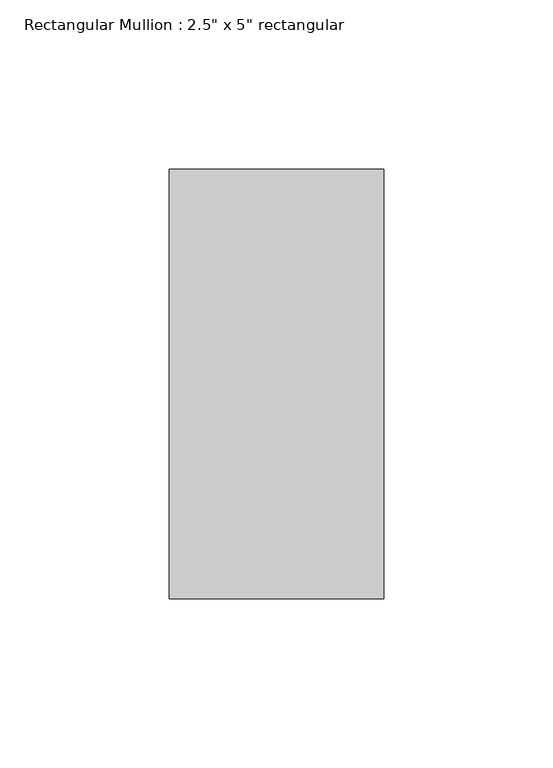
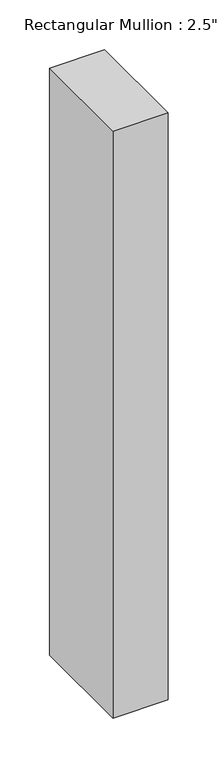
"""IFC4 building model written with IfcOpenShell, lengths in millimetres: member geometry."""

from ifc_helpers import new_model, si_unit, frame, origin, place, context, project, spatial, polyline, outline, extrude, source, transform, mapped, element, save


def member_c8ba4a72(model_context):
    return source(origin(), model_context, "Body", "SweptSolid", [
        extrude(outline(polyline([(31.75, 63.5), (31.75, -63.5), (-31.75, -63.5), (-31.75, 63.5), (31.75, 63.5)])), frame((0.0, 0.0, -717.5668761), z_axis=(0.0, 0.0, 1.0), x_axis=(1.0, 0.0, 0.0)), (0.0, 0.0, 1.0), 717.5668761),
    ])


if __name__ == "__main__":
    model = new_model("IFC4")
    model_context = context("Model", 3, world=origin())
    ifc_project = project(units=[si_unit("LENGTHUNIT", "METRE", prefix="MILLI")], contexts=[model_context])
    site = spatial("IfcSite", under=ifc_project)
    building = spatial("IfcBuilding", under=site)
    placement = place(None, origin())
    member_shape = member_c8ba4a72(model_context)
    element("IfcMember", 1, ObjectType="Rectangular Mullion : 2.5\" x 5\" rectangular", at=placement, inside=building, context=model_context, shape_type="MappedRepresentation", body=[
        mapped(member_shape, transform((0.0, 0.0, 0.0), x_axis=(1.0, 0.0, 0.0), y_axis=(0.0, 1.0, 0.0), z_axis=(0.0, 0.0, 1.0))),
    ])
    save(model, "model.ifc")

# Revit data of these elements
# Type "Rectangular Mullion : 2.5\" x 5\" rectangular"
#   built-in parameter 1007304 = 0.416667 (stored number, unit not read)
#   built-in parameter 1007301 = 0.104167 (stored number, unit not read)
#   built-in parameter 1007300 = 0.104167 (stored number, unit not read)
# Element 1 (IfcMember, "Rectangular Mullion : 2.5\" x 5\" rectangular")
#   Materials on its faces: "Aluminum"
# Materials
#   "Aluminum": class "Metal", colour RGB 247 247 247, transparency 0, Description = "Aluminum 6061", Cost = 0
